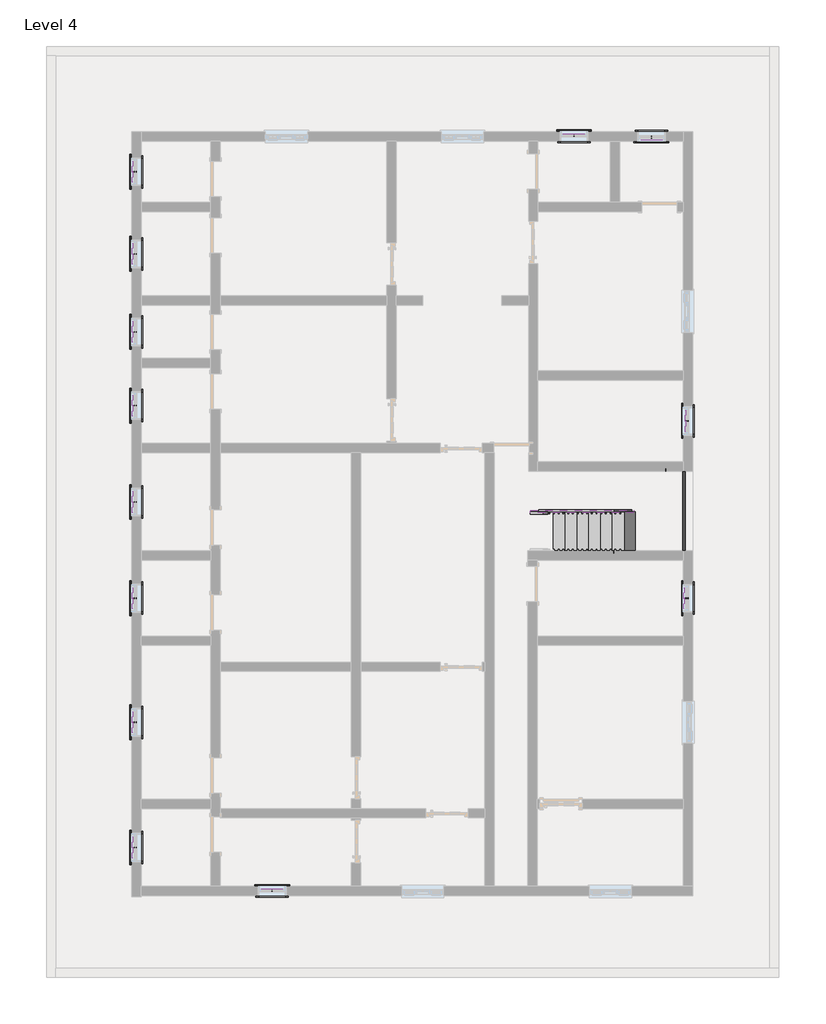
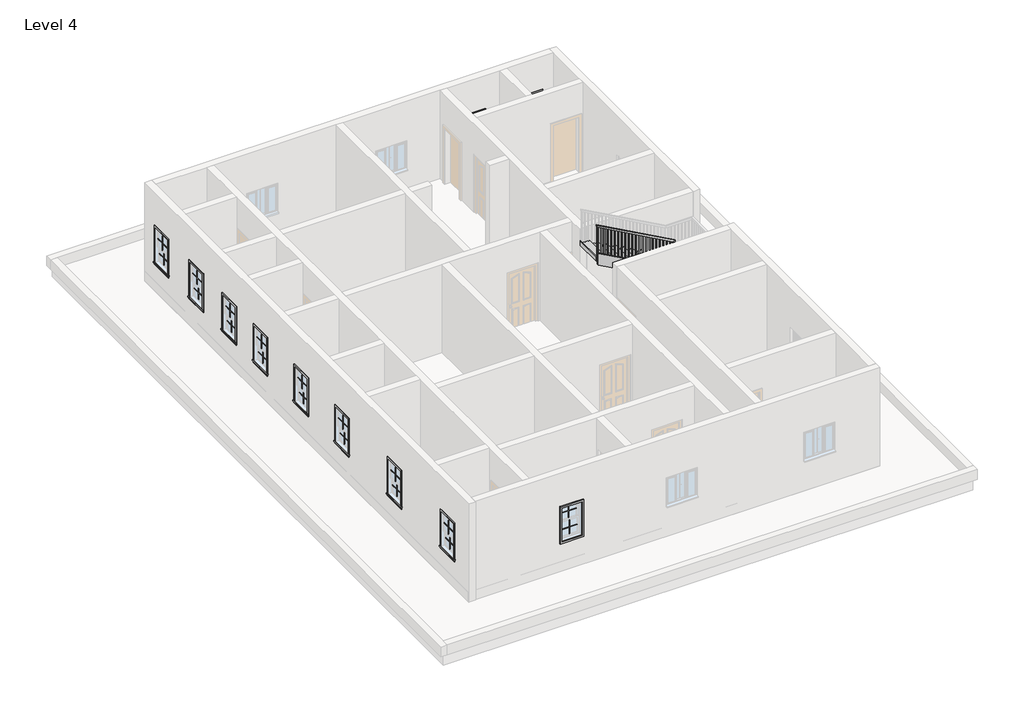
# One storey, part 3 of 3: 52 proxies, 5 members, 1 railing, 1 stair flight.
"""IFC4 building model written with IfcOpenShell, lengths in millimetres."""

from ifc_helpers import new_model, si_unit, frame, origin, place, context, project, spatial, polyline, outline, extrude, faceted_brep, transform, mapped, element, save
from components import muntin_pattern_2x2_muntin_pattern_2x2_eba6c5fb, trim_window_exterior_flat_with_sill_278e6a94, trim_window_interior_flat_picture_frame_e9fd5f45, stair_flight_f099b86a

model = new_model("IFC4")

# Units and contexts
model_context = context("Model", 3, world=origin())
ifc_project = project(units=[si_unit("LENGTHUNIT", "METRE", prefix="MILLI")], contexts=[model_context])

# Site, building, storey
site = spatial("IfcSite", under=ifc_project)
building = spatial("IfcBuilding", under=site)
storey = spatial("IfcBuildingStorey", under=building, Name="Level 4", Elevation=9144.0)

# Proxies
placement = place(None, origin())
muntin_pattern_2x2_muntin_pattern_2x2_shape = muntin_pattern_2x2_muntin_pattern_2x2_eba6c5fb(model_context)
element("IfcBuildingElementProxy", 1, Name="Muntin Pattern_2x2 : Muntin Pattern_2x2", ObjectType="Muntin Pattern_2x2 : Muntin Pattern_2x2", at=placement, inside=storey, context=model_context, shape_type="MappedRepresentation", body=[
    mapped(muntin_pattern_2x2_muntin_pattern_2x2_shape, transform((-10440.7626145, 6547.3404944, 10614.025), x_axis=(0.0, 1.0, 0.0), y_axis=(-1.0, 0.0, 0.0), z_axis=(0.0, 0.0, 1.0))),
])
element("IfcBuildingElementProxy", 2, Name="Muntin Pattern_2x2 : Muntin Pattern_2x2", ObjectType="Muntin Pattern_2x2 : Muntin Pattern_2x2", at=placement, inside=storey, context=model_context, shape_type="MappedRepresentation", body=[
    mapped(muntin_pattern_2x2_muntin_pattern_2x2_shape, transform((-10396.3126145, 6547.3404944, 10134.6), x_axis=(0.0, 1.0, 0.0), y_axis=(-1.0, 0.0, 0.0), z_axis=(0.0, 0.0, 1.0))),
])
element("IfcBuildingElementProxy", 3, Name="Muntin Pattern_2x2 : Muntin Pattern_2x2", ObjectType="Muntin Pattern_2x2 : Muntin Pattern_2x2", at=placement, inside=storey, context=model_context, shape_type="MappedRepresentation", body=[
    mapped(muntin_pattern_2x2_muntin_pattern_2x2_shape, transform((-10440.7626145, 4782.0404944, 10614.025), x_axis=(0.0, 1.0, 0.0), y_axis=(-1.0, 0.0, 0.0), z_axis=(0.0, 0.0, 1.0))),
])
element("IfcBuildingElementProxy", 4, Name="Muntin Pattern_2x2 : Muntin Pattern_2x2", ObjectType="Muntin Pattern_2x2 : Muntin Pattern_2x2", at=placement, inside=storey, context=model_context, shape_type="MappedRepresentation", body=[
    mapped(muntin_pattern_2x2_muntin_pattern_2x2_shape, transform((-10396.3126145, 4782.0404944, 10134.6), x_axis=(0.0, 1.0, 0.0), y_axis=(-1.0, 0.0, 0.0), z_axis=(0.0, 0.0, 1.0))),
])
element("IfcBuildingElementProxy", 5, Name="Muntin Pattern_2x2 : Muntin Pattern_2x2", ObjectType="Muntin Pattern_2x2 : Muntin Pattern_2x2", at=placement, inside=storey, context=model_context, shape_type="MappedRepresentation", body=[
    mapped(muntin_pattern_2x2_muntin_pattern_2x2_shape, transform((-10440.7626145, 3105.6404944, 10614.025), x_axis=(0.0, 1.0, 0.0), y_axis=(-1.0, 0.0, 0.0), z_axis=(0.0, 0.0, 1.0))),
])
element("IfcBuildingElementProxy", 6, Name="Muntin Pattern_2x2 : Muntin Pattern_2x2", ObjectType="Muntin Pattern_2x2 : Muntin Pattern_2x2", at=placement, inside=storey, context=model_context, shape_type="MappedRepresentation", body=[
    mapped(muntin_pattern_2x2_muntin_pattern_2x2_shape, transform((-10396.3126145, 3105.6404944, 10134.6), x_axis=(0.0, 1.0, 0.0), y_axis=(-1.0, 0.0, 0.0), z_axis=(0.0, 0.0, 1.0))),
])
element("IfcBuildingElementProxy", 7, Name="Muntin Pattern_2x2 : Muntin Pattern_2x2", ObjectType="Muntin Pattern_2x2 : Muntin Pattern_2x2", at=placement, inside=storey, context=model_context, shape_type="MappedRepresentation", body=[
    mapped(muntin_pattern_2x2_muntin_pattern_2x2_shape, transform((-10440.7626145, 1518.1404944, 10614.025), x_axis=(0.0, 1.0, 0.0), y_axis=(-1.0, 0.0, 0.0), z_axis=(0.0, 0.0, 1.0))),
])
element("IfcBuildingElementProxy", 8, Name="Muntin Pattern_2x2 : Muntin Pattern_2x2", ObjectType="Muntin Pattern_2x2 : Muntin Pattern_2x2", at=placement, inside=storey, context=model_context, shape_type="MappedRepresentation", body=[
    mapped(muntin_pattern_2x2_muntin_pattern_2x2_shape, transform((-10396.3126145, 1518.1404944, 10134.6), x_axis=(0.0, 1.0, 0.0), y_axis=(-1.0, 0.0, 0.0), z_axis=(0.0, 0.0, 1.0))),
])
element("IfcBuildingElementProxy", 9, Name="Muntin Pattern_2x2 : Muntin Pattern_2x2", ObjectType="Muntin Pattern_2x2 : Muntin Pattern_2x2", at=placement, inside=storey, context=model_context, shape_type="MappedRepresentation", body=[
    mapped(muntin_pattern_2x2_muntin_pattern_2x2_shape, transform((-10440.7626145, -551.9595056, 10614.025), x_axis=(0.0, 1.0, 0.0), y_axis=(-1.0, 0.0, 0.0), z_axis=(0.0, 0.0, 1.0))),
])
element("IfcBuildingElementProxy", 10, Name="Muntin Pattern_2x2 : Muntin Pattern_2x2", ObjectType="Muntin Pattern_2x2 : Muntin Pattern_2x2", at=placement, inside=storey, context=model_context, shape_type="MappedRepresentation", body=[
    mapped(muntin_pattern_2x2_muntin_pattern_2x2_shape, transform((-10396.3126145, -551.9595056, 10134.6), x_axis=(0.0, 1.0, 0.0), y_axis=(-1.0, 0.0, 0.0), z_axis=(0.0, 0.0, 1.0))),
])
element("IfcBuildingElementProxy", 11, Name="Muntin Pattern_2x2 : Muntin Pattern_2x2", ObjectType="Muntin Pattern_2x2 : Muntin Pattern_2x2", at=placement, inside=storey, context=model_context, shape_type="MappedRepresentation", body=[
    mapped(muntin_pattern_2x2_muntin_pattern_2x2_shape, transform((-10440.7626145, -2622.0595056, 10614.025), x_axis=(0.0, 1.0, 0.0), y_axis=(-1.0, 0.0, 0.0), z_axis=(0.0, 0.0, 1.0))),
])
element("IfcBuildingElementProxy", 12, Name="Muntin Pattern_2x2 : Muntin Pattern_2x2", ObjectType="Muntin Pattern_2x2 : Muntin Pattern_2x2", at=placement, inside=storey, context=model_context, shape_type="MappedRepresentation", body=[
    mapped(muntin_pattern_2x2_muntin_pattern_2x2_shape, transform((-10396.3126145, -2622.0595056, 10134.6), x_axis=(0.0, 1.0, 0.0), y_axis=(-1.0, 0.0, 0.0), z_axis=(0.0, 0.0, 1.0))),
])
element("IfcBuildingElementProxy", 13, Name="Muntin Pattern_2x2 : Muntin Pattern_2x2", ObjectType="Muntin Pattern_2x2 : Muntin Pattern_2x2", at=placement, inside=storey, context=model_context, shape_type="MappedRepresentation", body=[
    mapped(muntin_pattern_2x2_muntin_pattern_2x2_shape, transform((-10440.7626145, -5289.0595056, 10614.025), x_axis=(0.0, 1.0, 0.0), y_axis=(-1.0, 0.0, 0.0), z_axis=(0.0, 0.0, 1.0))),
])
element("IfcBuildingElementProxy", 14, Name="Muntin Pattern_2x2 : Muntin Pattern_2x2", ObjectType="Muntin Pattern_2x2 : Muntin Pattern_2x2", at=placement, inside=storey, context=model_context, shape_type="MappedRepresentation", body=[
    mapped(muntin_pattern_2x2_muntin_pattern_2x2_shape, transform((-10396.3126145, -5289.0595056, 10134.6), x_axis=(0.0, 1.0, 0.0), y_axis=(-1.0, 0.0, 0.0), z_axis=(0.0, 0.0, 1.0))),
])
element("IfcBuildingElementProxy", 15, Name="Muntin Pattern_2x2 : Muntin Pattern_2x2", ObjectType="Muntin Pattern_2x2 : Muntin Pattern_2x2", at=placement, inside=storey, context=model_context, shape_type="MappedRepresentation", body=[
    mapped(muntin_pattern_2x2_muntin_pattern_2x2_shape, transform((-10440.7626145, -7981.4595056, 10614.025), x_axis=(0.0, 1.0, 0.0), y_axis=(-1.0, 0.0, 0.0), z_axis=(0.0, 0.0, 1.0))),
])
element("IfcBuildingElementProxy", 16, Name="Muntin Pattern_2x2 : Muntin Pattern_2x2", ObjectType="Muntin Pattern_2x2 : Muntin Pattern_2x2", at=placement, inside=storey, context=model_context, shape_type="MappedRepresentation", body=[
    mapped(muntin_pattern_2x2_muntin_pattern_2x2_shape, transform((-10396.3126145, -7981.4595056, 10134.6), x_axis=(0.0, 1.0, 0.0), y_axis=(-1.0, 0.0, 0.0), z_axis=(0.0, 0.0, 1.0))),
])
element("IfcBuildingElementProxy", 17, Name="Muntin Pattern_2x2 : Muntin Pattern_2x2", ObjectType="Muntin Pattern_2x2 : Muntin Pattern_2x2", at=placement, inside=storey, context=model_context, shape_type="MappedRepresentation", body=[
    mapped(muntin_pattern_2x2_muntin_pattern_2x2_shape, transform((-7453.0876145, -8854.5845056, 10614.025), x_axis=(1.0, 0.0, 0.0), y_axis=(0.0, 1.0, 0.0), z_axis=(0.0, 0.0, 1.0))),
])
element("IfcBuildingElementProxy", 18, Name="Muntin Pattern_2x2 : Muntin Pattern_2x2", ObjectType="Muntin Pattern_2x2 : Muntin Pattern_2x2", at=placement, inside=storey, context=model_context, shape_type="MappedRepresentation", body=[
    mapped(muntin_pattern_2x2_muntin_pattern_2x2_shape, transform((-7453.0876145, -8899.0345056, 10134.6), x_axis=(1.0, 0.0, 0.0), y_axis=(0.0, 1.0, 0.0), z_axis=(0.0, 0.0, 1.0))),
])
element("IfcBuildingElementProxy", 19, Name="Muntin Pattern_2x2 : Muntin Pattern_2x2", ObjectType="Muntin Pattern_2x2 : Muntin Pattern_2x2", at=placement, inside=storey, context=model_context, shape_type="MappedRepresentation", body=[
    mapped(muntin_pattern_2x2_muntin_pattern_2x2_shape, transform((1421.0373855, -2622.0595056, 10614.025), x_axis=(0.0, 1.0, 0.0), y_axis=(-1.0, 0.0, 0.0), z_axis=(0.0, 0.0, 1.0))),
])
element("IfcBuildingElementProxy", 20, Name="Muntin Pattern_2x2 : Muntin Pattern_2x2", ObjectType="Muntin Pattern_2x2 : Muntin Pattern_2x2", at=placement, inside=storey, context=model_context, shape_type="MappedRepresentation", body=[
    mapped(muntin_pattern_2x2_muntin_pattern_2x2_shape, transform((1465.4873855, -2622.0595056, 10134.6), x_axis=(0.0, 1.0, 0.0), y_axis=(-1.0, 0.0, 0.0), z_axis=(0.0, 0.0, 1.0))),
])
element("IfcBuildingElementProxy", 21, Name="Muntin Pattern_2x2 : Muntin Pattern_2x2", ObjectType="Muntin Pattern_2x2 : Muntin Pattern_2x2", at=placement, inside=storey, context=model_context, shape_type="MappedRepresentation", body=[
    mapped(muntin_pattern_2x2_muntin_pattern_2x2_shape, transform((1421.0373855, 1190.4645364, 10614.025), x_axis=(0.0, 1.0, 0.0), y_axis=(-1.0, 0.0, 0.0), z_axis=(0.0, 0.0, 1.0))),
])
element("IfcBuildingElementProxy", 22, Name="Muntin Pattern_2x2 : Muntin Pattern_2x2", ObjectType="Muntin Pattern_2x2 : Muntin Pattern_2x2", at=placement, inside=storey, context=model_context, shape_type="MappedRepresentation", body=[
    mapped(muntin_pattern_2x2_muntin_pattern_2x2_shape, transform((1465.4873855, 1190.4645364, 10134.6), x_axis=(0.0, 1.0, 0.0), y_axis=(-1.0, 0.0, 0.0), z_axis=(0.0, 0.0, 1.0))),
])
element("IfcBuildingElementProxy", 23, Name="Muntin Pattern_2x2 : Muntin Pattern_2x2", ObjectType="Muntin Pattern_2x2 : Muntin Pattern_2x2", at=placement, inside=storey, context=model_context, shape_type="MappedRepresentation", body=[
    mapped(muntin_pattern_2x2_muntin_pattern_2x2_shape, transform((700.3123855, 7242.6654944, 10614.025), x_axis=(-1.0, 0.0, 0.0), y_axis=(0.0, -1.0, 0.0), z_axis=(0.0, 0.0, 1.0))),
])
element("IfcBuildingElementProxy", 24, Name="Muntin Pattern_2x2 : Muntin Pattern_2x2", ObjectType="Muntin Pattern_2x2 : Muntin Pattern_2x2", at=placement, inside=storey, context=model_context, shape_type="MappedRepresentation", body=[
    mapped(muntin_pattern_2x2_muntin_pattern_2x2_shape, transform((700.3123855, 7287.1154944, 10134.6), x_axis=(-1.0, 0.0, 0.0), y_axis=(0.0, -1.0, 0.0), z_axis=(0.0, 0.0, 1.0))),
])
element("IfcBuildingElementProxy", 25, Name="Muntin Pattern_2x2 : Muntin Pattern_2x2", ObjectType="Muntin Pattern_2x2 : Muntin Pattern_2x2", at=placement, inside=storey, context=model_context, shape_type="MappedRepresentation", body=[
    mapped(muntin_pattern_2x2_muntin_pattern_2x2_shape, transform((-963.3876145, 7376.0154944, 10614.025), x_axis=(1.0, 0.0, 0.0), y_axis=(0.0, 1.0, 0.0), z_axis=(0.0, 0.0, 1.0))),
])
element("IfcBuildingElementProxy", 26, Name="Muntin Pattern_2x2 : Muntin Pattern_2x2", ObjectType="Muntin Pattern_2x2 : Muntin Pattern_2x2", at=placement, inside=storey, context=model_context, shape_type="MappedRepresentation", body=[
    mapped(muntin_pattern_2x2_muntin_pattern_2x2_shape, transform((-963.3876145, 7331.5654944, 10134.6), x_axis=(1.0, 0.0, 0.0), y_axis=(0.0, 1.0, 0.0), z_axis=(0.0, 0.0, 1.0))),
])
trim_window_exterior_flat_with_sill_shape = trim_window_exterior_flat_with_sill_278e6a94(model_context)
element("IfcBuildingElementProxy", 27, Name="Trim-Window-Exterior-Flat : with Sill", ObjectType="Trim-Window-Exterior-Flat : with Sill", at=placement, inside=storey, context=model_context, shape_type="MappedRepresentation", body=[
    mapped(trim_window_exterior_flat_with_sill_shape, transform((-10475.6876145, 6547.3404944, 11125.2), x_axis=(0.0, -1.0, 0.0), y_axis=(0.0, 0.0, 1.0), z_axis=(-1.0, 0.0, 0.0))),
])
element("IfcBuildingElementProxy", 28, Name="Trim-Window-Exterior-Flat : with Sill", ObjectType="Trim-Window-Exterior-Flat : with Sill", at=placement, inside=storey, context=model_context, shape_type="MappedRepresentation", body=[
    mapped(trim_window_exterior_flat_with_sill_shape, transform((-10475.6876145, 4782.0404944, 11125.2), x_axis=(0.0, -1.0, 0.0), y_axis=(0.0, 0.0, 1.0), z_axis=(-1.0, 0.0, 0.0))),
])
element("IfcBuildingElementProxy", 29, Name="Trim-Window-Exterior-Flat : with Sill", ObjectType="Trim-Window-Exterior-Flat : with Sill", at=placement, inside=storey, context=model_context, shape_type="MappedRepresentation", body=[
    mapped(trim_window_exterior_flat_with_sill_shape, transform((-10475.6876145, 3105.6404944, 11125.2), x_axis=(0.0, -1.0, 0.0), y_axis=(0.0, 0.0, 1.0), z_axis=(-1.0, 0.0, 0.0))),
])
element("IfcBuildingElementProxy", 30, Name="Trim-Window-Exterior-Flat : with Sill", ObjectType="Trim-Window-Exterior-Flat : with Sill", at=placement, inside=storey, context=model_context, shape_type="MappedRepresentation", body=[
    mapped(trim_window_exterior_flat_with_sill_shape, transform((-10475.6876145, 1518.1404944, 11125.2), x_axis=(0.0, -1.0, 0.0), y_axis=(0.0, 0.0, 1.0), z_axis=(-1.0, 0.0, 0.0))),
])
element("IfcBuildingElementProxy", 31, Name="Trim-Window-Exterior-Flat : with Sill", ObjectType="Trim-Window-Exterior-Flat : with Sill", at=placement, inside=storey, context=model_context, shape_type="MappedRepresentation", body=[
    mapped(trim_window_exterior_flat_with_sill_shape, transform((-10475.6876145, -551.9595056, 11125.2), x_axis=(0.0, -1.0, 0.0), y_axis=(0.0, 0.0, 1.0), z_axis=(-1.0, 0.0, 0.0))),
])
element("IfcBuildingElementProxy", 32, Name="Trim-Window-Exterior-Flat : with Sill", ObjectType="Trim-Window-Exterior-Flat : with Sill", at=placement, inside=storey, context=model_context, shape_type="MappedRepresentation", body=[
    mapped(trim_window_exterior_flat_with_sill_shape, transform((-10475.6876145, -2622.0595056, 11125.2), x_axis=(0.0, -1.0, 0.0), y_axis=(0.0, 0.0, 1.0), z_axis=(-1.0, 0.0, 0.0))),
])
element("IfcBuildingElementProxy", 33, Name="Trim-Window-Exterior-Flat : with Sill", ObjectType="Trim-Window-Exterior-Flat : with Sill", at=placement, inside=storey, context=model_context, shape_type="MappedRepresentation", body=[
    mapped(trim_window_exterior_flat_with_sill_shape, transform((-10475.6876145, -5289.0595056, 11125.2), x_axis=(0.0, -1.0, 0.0), y_axis=(0.0, 0.0, 1.0), z_axis=(-1.0, 0.0, 0.0))),
])
element("IfcBuildingElementProxy", 34, Name="Trim-Window-Exterior-Flat : with Sill", ObjectType="Trim-Window-Exterior-Flat : with Sill", at=placement, inside=storey, context=model_context, shape_type="MappedRepresentation", body=[
    mapped(trim_window_exterior_flat_with_sill_shape, transform((-10475.6876145, -7981.4595056, 11125.2), x_axis=(0.0, -1.0, 0.0), y_axis=(0.0, 0.0, 1.0), z_axis=(-1.0, 0.0, 0.0))),
])
element("IfcBuildingElementProxy", 35, Name="Trim-Window-Exterior-Flat : with Sill", ObjectType="Trim-Window-Exterior-Flat : with Sill", at=placement, inside=storey, context=model_context, shape_type="MappedRepresentation", body=[
    mapped(trim_window_exterior_flat_with_sill_shape, transform((-7453.0876145, -8819.6595056, 11125.2), x_axis=(-1.0, 0.0, 0.0), y_axis=(0.0, 0.0, 1.0), z_axis=(0.0, 1.0, 0.0))),
])
element("IfcBuildingElementProxy", 36, Name="Trim-Window-Exterior-Flat : with Sill", ObjectType="Trim-Window-Exterior-Flat : with Sill", at=placement, inside=storey, context=model_context, shape_type="MappedRepresentation", body=[
    mapped(trim_window_exterior_flat_with_sill_shape, transform((1386.1123855, -2622.0595056, 11125.2), x_axis=(0.0, -1.0, 0.0), y_axis=(0.0, 0.0, 1.0), z_axis=(-1.0, 0.0, 0.0))),
])
element("IfcBuildingElementProxy", 37, Name="Trim-Window-Exterior-Flat : with Sill", ObjectType="Trim-Window-Exterior-Flat : with Sill", at=placement, inside=storey, context=model_context, shape_type="MappedRepresentation", body=[
    mapped(trim_window_exterior_flat_with_sill_shape, transform((1386.1123855, 1190.4645364, 11125.2), x_axis=(0.0, -1.0, 0.0), y_axis=(0.0, 0.0, 1.0), z_axis=(-1.0, 0.0, 0.0))),
])
element("IfcBuildingElementProxy", 38, Name="Trim-Window-Exterior-Flat : with Sill", ObjectType="Trim-Window-Exterior-Flat : with Sill", at=placement, inside=storey, context=model_context, shape_type="MappedRepresentation", body=[
    mapped(trim_window_exterior_flat_with_sill_shape, transform((700.3123855, 7207.7404944, 11125.2), x_axis=(1.0, 0.0, 0.0), y_axis=(0.0, 0.0, 1.0), z_axis=(0.0, -1.0, 0.0))),
])
element("IfcBuildingElementProxy", 39, Name="Trim-Window-Exterior-Flat : with Sill", ObjectType="Trim-Window-Exterior-Flat : with Sill", at=placement, inside=storey, context=model_context, shape_type="MappedRepresentation", body=[
    mapped(trim_window_exterior_flat_with_sill_shape, transform((-963.3876145, 7410.9404944, 11125.2), x_axis=(-1.0, 0.0, 0.0), y_axis=(0.0, 0.0, 1.0), z_axis=(0.0, 1.0, 0.0))),
])
trim_window_interior_flat_picture_frame_shape = trim_window_interior_flat_picture_frame_e9fd5f45(model_context)
element("IfcBuildingElementProxy", 40, Name="Trim-Window-Interior-Flat : Picture Frame", ObjectType="Trim-Window-Interior-Flat : Picture Frame", at=placement, inside=storey, context=model_context, shape_type="MappedRepresentation", body=[
    mapped(trim_window_interior_flat_picture_frame_shape, transform((-10272.4876145, 6547.3404944, 11125.2), x_axis=(0.0, 1.0, 0.0), y_axis=(0.0, 0.0, 1.0), z_axis=(1.0, 0.0, 0.0))),
])
element("IfcBuildingElementProxy", 41, Name="Trim-Window-Interior-Flat : Picture Frame", ObjectType="Trim-Window-Interior-Flat : Picture Frame", at=placement, inside=storey, context=model_context, shape_type="MappedRepresentation", body=[
    mapped(trim_window_interior_flat_picture_frame_shape, transform((-10272.4876145, 4782.0404944, 11125.2), x_axis=(0.0, 1.0, 0.0), y_axis=(0.0, 0.0, 1.0), z_axis=(1.0, 0.0, 0.0))),
])
element("IfcBuildingElementProxy", 42, Name="Trim-Window-Interior-Flat : Picture Frame", ObjectType="Trim-Window-Interior-Flat : Picture Frame", at=placement, inside=storey, context=model_context, shape_type="MappedRepresentation", body=[
    mapped(trim_window_interior_flat_picture_frame_shape, transform((-10272.4876145, 3105.6404944, 11125.2), x_axis=(0.0, 1.0, 0.0), y_axis=(0.0, 0.0, 1.0), z_axis=(1.0, 0.0, 0.0))),
])
element("IfcBuildingElementProxy", 43, Name="Trim-Window-Interior-Flat : Picture Frame", ObjectType="Trim-Window-Interior-Flat : Picture Frame", at=placement, inside=storey, context=model_context, shape_type="MappedRepresentation", body=[
    mapped(trim_window_interior_flat_picture_frame_shape, transform((-10272.4876145, 1518.1404944, 11125.2), x_axis=(0.0, 1.0, 0.0), y_axis=(0.0, 0.0, 1.0), z_axis=(1.0, 0.0, 0.0))),
])
element("IfcBuildingElementProxy", 44, Name="Trim-Window-Interior-Flat : Picture Frame", ObjectType="Trim-Window-Interior-Flat : Picture Frame", at=placement, inside=storey, context=model_context, shape_type="MappedRepresentation", body=[
    mapped(trim_window_interior_flat_picture_frame_shape, transform((-10272.4876145, -551.9595056, 11125.2), x_axis=(0.0, 1.0, 0.0), y_axis=(0.0, 0.0, 1.0), z_axis=(1.0, 0.0, 0.0))),
])
element("IfcBuildingElementProxy", 45, Name="Trim-Window-Interior-Flat : Picture Frame", ObjectType="Trim-Window-Interior-Flat : Picture Frame", at=placement, inside=storey, context=model_context, shape_type="MappedRepresentation", body=[
    mapped(trim_window_interior_flat_picture_frame_shape, transform((-10272.4876145, -2622.0595056, 11125.2), x_axis=(0.0, 1.0, 0.0), y_axis=(0.0, 0.0, 1.0), z_axis=(1.0, 0.0, 0.0))),
])
element("IfcBuildingElementProxy", 46, Name="Trim-Window-Interior-Flat : Picture Frame", ObjectType="Trim-Window-Interior-Flat : Picture Frame", at=placement, inside=storey, context=model_context, shape_type="MappedRepresentation", body=[
    mapped(trim_window_interior_flat_picture_frame_shape, transform((-10272.4876145, -5289.0595056, 11125.2), x_axis=(0.0, 1.0, 0.0), y_axis=(0.0, 0.0, 1.0), z_axis=(1.0, 0.0, 0.0))),
])
element("IfcBuildingElementProxy", 47, Name="Trim-Window-Interior-Flat : Picture Frame", ObjectType="Trim-Window-Interior-Flat : Picture Frame", at=placement, inside=storey, context=model_context, shape_type="MappedRepresentation", body=[
    mapped(trim_window_interior_flat_picture_frame_shape, transform((-10272.4876145, -7981.4595056, 11125.2), x_axis=(0.0, 1.0, 0.0), y_axis=(0.0, 0.0, 1.0), z_axis=(1.0, 0.0, 0.0))),
])
element("IfcBuildingElementProxy", 48, Name="Trim-Window-Interior-Flat : Picture Frame", ObjectType="Trim-Window-Interior-Flat : Picture Frame", at=placement, inside=storey, context=model_context, shape_type="MappedRepresentation", body=[
    mapped(trim_window_interior_flat_picture_frame_shape, transform((-7453.0876145, -9022.8595056, 11125.2), x_axis=(1.0, 0.0, 0.0), y_axis=(0.0, 0.0, 1.0), z_axis=(0.0, -1.0, 0.0))),
])
element("IfcBuildingElementProxy", 49, Name="Trim-Window-Interior-Flat : Picture Frame", ObjectType="Trim-Window-Interior-Flat : Picture Frame", at=placement, inside=storey, context=model_context, shape_type="MappedRepresentation", body=[
    mapped(trim_window_interior_flat_picture_frame_shape, transform((1589.3123855, -2622.0595056, 11125.2), x_axis=(0.0, 1.0, 0.0), y_axis=(0.0, 0.0, 1.0), z_axis=(1.0, 0.0, 0.0))),
])
element("IfcBuildingElementProxy", 50, Name="Trim-Window-Interior-Flat : Picture Frame", ObjectType="Trim-Window-Interior-Flat : Picture Frame", at=placement, inside=storey, context=model_context, shape_type="MappedRepresentation", body=[
    mapped(trim_window_interior_flat_picture_frame_shape, transform((1589.3123855, 1190.4645364, 11125.2), x_axis=(0.0, 1.0, 0.0), y_axis=(0.0, 0.0, 1.0), z_axis=(1.0, 0.0, 0.0))),
])
element("IfcBuildingElementProxy", 51, Name="Trim-Window-Interior-Flat : Picture Frame", ObjectType="Trim-Window-Interior-Flat : Picture Frame", at=placement, inside=storey, context=model_context, shape_type="MappedRepresentation", body=[
    mapped(trim_window_interior_flat_picture_frame_shape, transform((700.3123855, 7410.9404944, 11125.2), x_axis=(-1.0, 0.0, 0.0), y_axis=(0.0, 0.0, 1.0), z_axis=(0.0, 1.0, 0.0))),
])
element("IfcBuildingElementProxy", 52, Name="Trim-Window-Interior-Flat : Picture Frame", ObjectType="Trim-Window-Interior-Flat : Picture Frame", at=placement, inside=storey, context=model_context, shape_type="MappedRepresentation", body=[
    mapped(trim_window_interior_flat_picture_frame_shape, transform((-963.3876145, 7207.7404944, 11125.2), x_axis=(1.0, 0.0, 0.0), y_axis=(0.0, 0.0, 1.0), z_axis=(0.0, -1.0, 0.0))),
])

# Members
element("IfcMember", 53, ObjectType="Stringer - 2\" Width", at=placement, inside=storey, context=model_context, shape_type="SweptSolid", body=[
    extrude(outline(polyline([(9354.6757607, -1903.1876145), (9144.0, -1903.1876145), (9144.0, -1654.2050647), (10209.4963497, 274.6830625), (10557.7073019, 274.6830625), (9354.6757607, -1903.1876145)])), frame((0.0, -767.8595056, 0.0), z_axis=(0.0, 1.0, 0.0), x_axis=(0.0, 0.0, 1.0)), (0.0, 0.0, 1.0), 50.8),
])
element("IfcMember", 54, ObjectType="Stringer - 2\" Width", at=placement, inside=storey, context=model_context, shape_type="SweptSolid", body=[
    extrude(outline(polyline([(10374.7177047, 325.4830625), (10722.928657, 325.4830625), (11954.0215532, -1903.1876145), (11605.8106009, -1903.1876145), (10374.7177047, 325.4830625)])), frame((0.0, -780.5595056, 0.0), z_axis=(0.0, 1.0, 0.0), x_axis=(0.0, 0.0, 1.0)), (0.0, 0.0, 1.0), 50.8),
])
element("IfcMember", 55, ObjectType="Stringer - 2\" Width", at=placement, inside=storey, context=model_context, shape_type="SweptSolid", body=[
    extrude(outline(polyline([(9354.6757607, -1903.1876145), (9144.0, -1903.1876145), (9144.0, -1654.2050647), (10591.8, 966.7745674), (10591.8, 336.4017165), (9354.6757607, -1903.1876145)])), frame((0.0, -1656.8595056, 0.0), z_axis=(0.0, 1.0, 0.0), x_axis=(0.0, 0.0, 1.0)), (0.0, 0.0, 1.0), 50.8),
])
element("IfcMember", 56, ObjectType="Stringer - 2\" Width", at=placement, inside=storey, context=model_context, shape_type="SweptSolid", body=[
    extrude(outline(polyline([(1424.2123855, -1656.8595056), (1373.4123855, -1656.8595056), (1373.4123855, 108.4404944), (1424.2123855, 108.4404944), (1424.2123855, -1656.8595056)])), frame((0.0, 0.0, 10287.0), z_axis=(0.0, 0.0, 1.0), x_axis=(1.0, 0.0, 0.0)), (0.0, 0.0, 1.0), 304.8),
])
element("IfcMember", 57, ObjectType="Stringer - 2\" Width", at=placement, inside=storey, context=model_context, shape_type="SweptSolid", body=[
    extrude(outline(polyline([(10287.0, 1114.6529278), (11954.0215532, -1903.1876145), (11605.8106009, -1903.1876145), (10287.0, 484.2800769), (10287.0, 1114.6529278)])), frame((0.0, 108.4404944, 0.0), z_axis=(0.0, 1.0, 0.0), x_axis=(0.0, 0.0, 1.0)), (0.0, 0.0, 1.0), 50.8),
])

# Railing
element("IfcRailing", 58, ObjectType="Handrail - Rectangular", at=placement, inside=storey, context=model_context, shape_type="SolidModel", body=[
    faceted_brep([(-1903.1876145, -767.8595056, 10195.56), (-1903.1876145, -767.8595056, 10137.4879132), (-1903.1876145, -818.6595056, 10137.4879132), (-1903.1876145, -818.6595056, 10195.56), (325.4830625, -767.8595056, 11430.0), (325.4830625, -818.6595056, 11430.0), (325.4830625, -818.6595056, 11371.9279132), (325.4830625, -767.8595056, 11371.9279132)], [[[0, 1, 2, 3]], [[4, 5, 6, 7]], [[1, 0, 4, 7]], [[2, 1, 7, 6]], [[3, 2, 6, 5]], [[0, 3, 5, 4]]]),
    faceted_brep([(325.4830625, -818.6595056, 11430.0), (325.4830625, -818.6595056, 11379.2), (376.2830625, -818.6595056, 11379.2), (376.2830625, -818.6595056, 11430.0), (325.4830625, -729.7595056, 11430.0), (376.2830625, -729.7595056, 11430.0), (376.2830625, -678.9595056, 11379.2), (325.4830625, -678.9595056, 11379.2)], [[[0, 1, 2, 3]], [[4, 5, 6, 7]], [[1, 0, 4, 7]], [[2, 1, 7, 6]], [[3, 2, 6, 5]], [[0, 3, 5, 4]]]),
    faceted_brep([(325.4830625, -729.7595056, 11430.0), (325.4830625, -678.9595056, 11379.2), (376.2830625, -678.9595056, 11379.2), (376.2830625, -729.7595056, 11430.0), (325.4830625, -729.7595056, 11509.0879132), (376.2830625, -729.7595056, 11539.0223516), (376.2830625, -678.9595056, 11539.0223516), (325.4830625, -678.9595056, 11509.0879132)], [[[0, 1, 2, 3]], [[4, 5, 6, 7]], [[1, 0, 4, 7]], [[2, 1, 7, 6]], [[3, 2, 6, 5]], [[0, 3, 5, 4]]]),
    faceted_brep([(376.2830625, -729.7595056, 11539.0223516), (325.4830625, -729.7595056, 11509.0879132), (325.4830625, -678.9595056, 11509.0879132), (376.2830625, -678.9595056, 11539.0223516), (-1903.1876145, -729.7595056, 12801.6), (-1903.1876145, -678.9595056, 12801.6), (-1903.1876145, -678.9595056, 12743.5279132), (-1903.1876145, -729.7595056, 12743.5279132)], [[[0, 1, 2, 3]], [[4, 5, 6, 7]], [[1, 0, 4, 7]], [[2, 1, 7, 6]], [[3, 2, 6, 5]], [[0, 3, 5, 4]]]),
    extrude(outline(polyline([(12738.3072849, -1893.8419375), (11750.04, -1893.8419375), (11750.04, -1874.7919375), (12727.7556667, -1874.7919375), (12738.3072849, -1893.8419375)])), frame((0.0, -713.8845056, 0.0), z_axis=(0.0, 1.0, 0.0), x_axis=(0.0, 0.0, 1.0)), (0.0, 0.0, 1.0), 19.05),
    extrude(outline(polyline([(12682.031988, -1792.2419375), (11750.04, -1792.2419375), (11750.04, -1773.1919375), (12671.4803699, -1773.1919375), (12682.031988, -1792.2419375)])), frame((0.0, -713.8845056, 0.0), z_axis=(0.0, 1.0, 0.0), x_axis=(0.0, 0.0, 1.0)), (0.0, 0.0, 1.0), 19.05),
    extrude(outline(polyline([(12625.7125465, -1690.6419375), (11750.04, -1690.6419375), (11750.04, -1671.5919375), (12615.1609284, -1671.5919375), (12625.7125465, -1690.6419375)])), frame((0.0, -713.8845056, 0.0), z_axis=(0.0, 1.0, 0.0), x_axis=(0.0, 0.0, 1.0)), (0.0, 0.0, 1.0), 19.05),
    extrude(outline(polyline([(12569.4813943, -1589.0419375), (11612.88, -1589.0419375), (11612.88, -1569.9919375), (12558.9297761, -1569.9919375), (12569.4813943, -1589.0419375)])), frame((0.0, -713.8845056, 0.0), z_axis=(0.0, 1.0, 0.0), x_axis=(0.0, 0.0, 1.0)), (0.0, 0.0, 1.0), 19.05),
    extrude(outline(polyline([(12513.2060974, -1487.4419375), (11612.88, -1487.4419375), (11612.88, -1468.3919375), (12502.6544792, -1468.3919375), (12513.2060974, -1487.4419375)])), frame((0.0, -713.8845056, 0.0), z_axis=(0.0, 1.0, 0.0), x_axis=(0.0, 0.0, 1.0)), (0.0, 0.0, 1.0), 19.05),
    extrude(outline(polyline([(12456.9308005, -1385.8419375), (11475.72, -1385.8419375), (11475.72, -1366.7919375), (12446.3791823, -1366.7919375), (12456.9308005, -1385.8419375)])), frame((0.0, -713.8845056, 0.0), z_axis=(0.0, 1.0, 0.0), x_axis=(0.0, 0.0, 1.0)), (0.0, 0.0, 1.0), 19.05),
    extrude(outline(polyline([(12400.6555036, -1284.2419375), (11475.72, -1284.2419375), (11475.72, -1265.1919375), (12390.1038855, -1265.1919375), (12400.6555036, -1284.2419375)])), frame((0.0, -713.8845056, 0.0), z_axis=(0.0, 1.0, 0.0), x_axis=(0.0, 0.0, 1.0)), (0.0, 0.0, 1.0), 19.05),
    extrude(outline(polyline([(12344.3802067, -1182.6419375), (11475.72, -1182.6419375), (11475.72, -1163.5919375), (12333.8285886, -1163.5919375), (12344.3802067, -1182.6419375)])), frame((0.0, -713.8845056, 0.0), z_axis=(0.0, 1.0, 0.0), x_axis=(0.0, 0.0, 1.0)), (0.0, 0.0, 1.0), 19.05),
    extrude(outline(polyline([(12288.1049099, -1081.0419375), (11338.56, -1081.0419375), (11338.56, -1061.9919375), (12277.5532917, -1061.9919375), (12288.1049099, -1081.0419375)])), frame((0.0, -713.8845056, 0.0), z_axis=(0.0, 1.0, 0.0), x_axis=(0.0, 0.0, 1.0)), (0.0, 0.0, 1.0), 19.05),
    extrude(outline(polyline([(12231.829613, -979.4419375), (11338.56, -979.4419375), (11338.56, -960.3919375), (12221.2779948, -960.3919375), (12231.829613, -979.4419375)])), frame((0.0, -713.8845056, 0.0), z_axis=(0.0, 1.0, 0.0), x_axis=(0.0, 0.0, 1.0)), (0.0, 0.0, 1.0), 19.05),
    extrude(outline(polyline([(12175.5543161, -877.8419375), (11201.4, -877.8419375), (11201.4, -858.7919375), (12165.0026979, -858.7919375), (12175.5543161, -877.8419375)])), frame((0.0, -713.8845056, 0.0), z_axis=(0.0, 1.0, 0.0), x_axis=(0.0, 0.0, 1.0)), (0.0, 0.0, 1.0), 19.05),
    extrude(outline(polyline([(12119.2790192, -776.2419375), (11201.4, -776.2419375), (11201.4, -757.1919375), (12108.727401, -757.1919375), (12119.2790192, -776.2419375)])), frame((0.0, -713.8845056, 0.0), z_axis=(0.0, 1.0, 0.0), x_axis=(0.0, 0.0, 1.0)), (0.0, 0.0, 1.0), 19.05),
    extrude(outline(polyline([(12063.0478669, -674.6419375), (11201.4, -674.6419375), (11201.4, -655.5919375), (12052.4962488, -655.5919375), (12063.0478669, -674.6419375)])), frame((0.0, -713.8845056, 0.0), z_axis=(0.0, 1.0, 0.0), x_axis=(0.0, 0.0, 1.0)), (0.0, 0.0, 1.0), 19.05),
    extrude(outline(polyline([(12006.77257, -573.0419375), (11064.24, -573.0419375), (11064.24, -553.9919375), (11996.2209519, -553.9919375), (12006.77257, -573.0419375)])), frame((0.0, -713.8845056, 0.0), z_axis=(0.0, 1.0, 0.0), x_axis=(0.0, 0.0, 1.0)), (0.0, 0.0, 1.0), 19.05),
    extrude(outline(polyline([(11950.4972732, -471.4419375), (11064.24, -471.4419375), (11064.24, -452.3919375), (11939.945655, -452.3919375), (11950.4972732, -471.4419375)])), frame((0.0, -713.8845056, 0.0), z_axis=(0.0, 1.0, 0.0), x_axis=(0.0, 0.0, 1.0)), (0.0, 0.0, 1.0), 19.05),
    extrude(outline(polyline([(11894.2219763, -369.8419375), (10927.08, -369.8419375), (10927.08, -350.7919375), (11883.6703581, -350.7919375), (11894.2219763, -369.8419375)])), frame((0.0, -713.8845056, 0.0), z_axis=(0.0, 1.0, 0.0), x_axis=(0.0, 0.0, 1.0)), (0.0, 0.0, 1.0), 19.05),
    extrude(outline(polyline([(11837.9466794, -268.2419375), (10927.08, -268.2419375), (10927.08, -249.1919375), (11827.3950612, -249.1919375), (11837.9466794, -268.2419375)])), frame((0.0, -713.8845056, 0.0), z_axis=(0.0, 1.0, 0.0), x_axis=(0.0, 0.0, 1.0)), (0.0, 0.0, 1.0), 19.05),
    extrude(outline(polyline([(11781.6713825, -166.6419375), (10927.08, -166.6419375), (10927.08, -147.5919375), (11771.1197643, -147.5919375), (11781.6713825, -166.6419375)])), frame((0.0, -713.8845056, 0.0), z_axis=(0.0, 1.0, 0.0), x_axis=(0.0, 0.0, 1.0)), (0.0, 0.0, 1.0), 19.05),
    extrude(outline(polyline([(11725.3960856, -65.0419375), (10789.92, -65.0419375), (10789.92, -45.9919375), (11714.8444675, -45.9919375), (11725.3960856, -65.0419375)])), frame((0.0, -713.8845056, 0.0), z_axis=(0.0, 1.0, 0.0), x_axis=(0.0, 0.0, 1.0)), (0.0, 0.0, 1.0), 19.05),
    extrude(outline(polyline([(11669.1207888, 36.5580625), (10789.92, 36.5580625), (10789.92, 55.6080625), (11658.5691706, 55.6080625), (11669.1207888, 36.5580625)])), frame((0.0, -713.8845056, 0.0), z_axis=(0.0, 1.0, 0.0), x_axis=(0.0, 0.0, 1.0)), (0.0, 0.0, 1.0), 19.05),
    extrude(outline(polyline([(11612.8454919, 138.1580625), (10652.76, 138.1580625), (10652.76, 157.2080625), (11602.2938737, 157.2080625), (11612.8454919, 138.1580625)])), frame((0.0, -713.8845056, 0.0), z_axis=(0.0, 1.0, 0.0), x_axis=(0.0, 0.0, 1.0)), (0.0, 0.0, 1.0), 19.05),
    extrude(outline(polyline([(11556.570195, 239.7580625), (10652.76, 239.7580625), (10652.76, 258.8080625), (11546.0185768, 258.8080625), (11556.570195, 239.7580625)])), frame((0.0, -713.8845056, 0.0), z_axis=(0.0, 1.0, 0.0), x_axis=(0.0, 0.0, 1.0)), (0.0, 0.0, 1.0), 19.05),
    extrude(outline(polyline([(11370.2686355, 322.4873855), (10515.6, 322.4873855), (10515.6, 341.5373855), (11380.8202537, 341.5373855), (11370.2686355, 322.4873855)])), frame((0.0, -802.7845056, 0.0), z_axis=(0.0, 1.0, 0.0), x_axis=(0.0, 0.0, 1.0)), (0.0, 0.0, 1.0), 19.05),
    extrude(outline(polyline([(11313.9933387, 220.8873855), (10378.44, 220.8873855), (10378.44, 239.9373855), (11324.5449568, 239.9373855), (11313.9933387, 220.8873855)])), frame((0.0, -802.7845056, 0.0), z_axis=(0.0, 1.0, 0.0), x_axis=(0.0, 0.0, 1.0)), (0.0, 0.0, 1.0), 19.05),
    extrude(outline(polyline([(11257.7180418, 119.2873855), (10378.44, 119.2873855), (10378.44, 138.3373855), (11268.2696599, 138.3373855), (11257.7180418, 119.2873855)])), frame((0.0, -802.7845056, 0.0), z_axis=(0.0, 1.0, 0.0), x_axis=(0.0, 0.0, 1.0)), (0.0, 0.0, 1.0), 19.05),
    extrude(outline(polyline([(11201.4427449, 17.6873855), (10241.28, 17.6873855), (10241.28, 36.7373855), (11211.9943631, 36.7373855), (11201.4427449, 17.6873855)])), frame((0.0, -802.7845056, 0.0), z_axis=(0.0, 1.0, 0.0), x_axis=(0.0, 0.0, 1.0)), (0.0, 0.0, 1.0), 19.05),
    extrude(outline(polyline([(11145.167448, -83.9126145), (10241.28, -83.9126145), (10241.28, -64.8626145), (11155.7190662, -64.8626145), (11145.167448, -83.9126145)])), frame((0.0, -802.7845056, 0.0), z_axis=(0.0, 1.0, 0.0), x_axis=(0.0, 0.0, 1.0)), (0.0, 0.0, 1.0), 19.05),
    extrude(outline(polyline([(11088.8921511, -185.5126145), (10104.12, -185.5126145), (10104.12, -166.4626145), (11099.4437693, -166.4626145), (11088.8921511, -185.5126145)])), frame((0.0, -802.7845056, 0.0), z_axis=(0.0, 1.0, 0.0), x_axis=(0.0, 0.0, 1.0)), (0.0, 0.0, 1.0), 19.05),
    extrude(outline(polyline([(11032.6168543, -287.1126145), (10104.12, -287.1126145), (10104.12, -268.0626145), (11043.1684724, -268.0626145), (11032.6168543, -287.1126145)])), frame((0.0, -802.7845056, 0.0), z_axis=(0.0, 1.0, 0.0), x_axis=(0.0, 0.0, 1.0)), (0.0, 0.0, 1.0), 19.05),
    extrude(outline(polyline([(10976.3415574, -388.7126145), (10104.12, -388.7126145), (10104.12, -369.6626145), (10986.8931755, -369.6626145), (10976.3415574, -388.7126145)])), frame((0.0, -802.7845056, 0.0), z_axis=(0.0, 1.0, 0.0), x_axis=(0.0, 0.0, 1.0)), (0.0, 0.0, 1.0), 19.05),
    extrude(outline(polyline([(10920.0662605, -490.3126145), (9966.96, -490.3126145), (9966.96, -471.2626145), (10930.6178787, -471.2626145), (10920.0662605, -490.3126145)])), frame((0.0, -802.7845056, 0.0), z_axis=(0.0, 1.0, 0.0), x_axis=(0.0, 0.0, 1.0)), (0.0, 0.0, 1.0), 19.05),
    extrude(outline(polyline([(10863.7909636, -591.9126145), (9966.96, -591.9126145), (9966.96, -572.8626145), (10874.3425818, -572.8626145), (10863.7909636, -591.9126145)])), frame((0.0, -802.7845056, 0.0), z_axis=(0.0, 1.0, 0.0), x_axis=(0.0, 0.0, 1.0)), (0.0, 0.0, 1.0), 19.05),
    extrude(outline(polyline([(10807.5156667, -693.5126145), (9829.8, -693.5126145), (9829.8, -674.4626145), (10818.0672849, -674.4626145), (10807.5156667, -693.5126145)])), frame((0.0, -802.7845056, 0.0), z_axis=(0.0, 1.0, 0.0), x_axis=(0.0, 0.0, 1.0)), (0.0, 0.0, 1.0), 19.05),
    extrude(outline(polyline([(10751.2403699, -795.1126145), (9829.8, -795.1126145), (9829.8, -776.0626145), (10761.791988, -776.0626145), (10751.2403699, -795.1126145)])), frame((0.0, -802.7845056, 0.0), z_axis=(0.0, 1.0, 0.0), x_axis=(0.0, 0.0, 1.0)), (0.0, 0.0, 1.0), 19.05),
    extrude(outline(polyline([(10694.9209284, -896.7126145), (9829.8, -896.7126145), (9829.8, -877.6626145), (10705.4725466, -877.6626145), (10694.9209284, -896.7126145)])), frame((0.0, -802.7845056, 0.0), z_axis=(0.0, 1.0, 0.0), x_axis=(0.0, 0.0, 1.0)), (0.0, 0.0, 1.0), 19.05),
    extrude(outline(polyline([(10638.6897761, -998.3126145), (9692.64, -998.3126145), (9692.64, -979.2626145), (10649.2413943, -979.2626145), (10638.6897761, -998.3126145)])), frame((0.0, -802.7845056, 0.0), z_axis=(0.0, 1.0, 0.0), x_axis=(0.0, 0.0, 1.0)), (0.0, 0.0, 1.0), 19.05),
    extrude(outline(polyline([(10582.4144792, -1099.9126145), (9692.64, -1099.9126145), (9692.64, -1080.8626145), (10592.9660974, -1080.8626145), (10582.4144792, -1099.9126145)])), frame((0.0, -802.7845056, 0.0), z_axis=(0.0, 1.0, 0.0), x_axis=(0.0, 0.0, 1.0)), (0.0, 0.0, 1.0), 19.05),
    extrude(outline(polyline([(10526.1391823, -1201.5126145), (9555.48, -1201.5126145), (9555.48, -1182.4626145), (10536.6908005, -1182.4626145), (10526.1391823, -1201.5126145)])), frame((0.0, -802.7845056, 0.0), z_axis=(0.0, 1.0, 0.0), x_axis=(0.0, 0.0, 1.0)), (0.0, 0.0, 1.0), 19.05),
    extrude(outline(polyline([(10469.8638855, -1303.1126145), (9555.48, -1303.1126145), (9555.48, -1284.0626145), (10480.4155036, -1284.0626145), (10469.8638855, -1303.1126145)])), frame((0.0, -802.7845056, 0.0), z_axis=(0.0, 1.0, 0.0), x_axis=(0.0, 0.0, 1.0)), (0.0, 0.0, 1.0), 19.05),
    extrude(outline(polyline([(10413.5885886, -1404.7126145), (9555.48, -1404.7126145), (9555.48, -1385.6626145), (10424.1402067, -1385.6626145), (10413.5885886, -1404.7126145)])), frame((0.0, -802.7845056, 0.0), z_axis=(0.0, 1.0, 0.0), x_axis=(0.0, 0.0, 1.0)), (0.0, 0.0, 1.0), 19.05),
    extrude(outline(polyline([(10357.3132917, -1506.3126145), (9418.32, -1506.3126145), (9418.32, -1487.2626145), (10367.8649099, -1487.2626145), (10357.3132917, -1506.3126145)])), frame((0.0, -802.7845056, 0.0), z_axis=(0.0, 1.0, 0.0), x_axis=(0.0, 0.0, 1.0)), (0.0, 0.0, 1.0), 19.05),
    extrude(outline(polyline([(10301.0379948, -1607.9126145), (9418.32, -1607.9126145), (9418.32, -1588.8626145), (10311.589613, -1588.8626145), (10301.0379948, -1607.9126145)])), frame((0.0, -802.7845056, 0.0), z_axis=(0.0, 1.0, 0.0), x_axis=(0.0, 0.0, 1.0)), (0.0, 0.0, 1.0), 19.05),
    extrude(outline(polyline([(10244.7626979, -1709.5126145), (9281.16, -1709.5126145), (9281.16, -1690.4626145), (10255.3143161, -1690.4626145), (10244.7626979, -1709.5126145)])), frame((0.0, -802.7845056, 0.0), z_axis=(0.0, 1.0, 0.0), x_axis=(0.0, 0.0, 1.0)), (0.0, 0.0, 1.0), 19.05),
    extrude(outline(polyline([(10188.487401, -1811.1126145), (9281.16, -1811.1126145), (9281.16, -1792.0626145), (10199.0390192, -1792.0626145), (10188.487401, -1811.1126145)])), frame((0.0, -802.7845056, 0.0), z_axis=(0.0, 1.0, 0.0), x_axis=(0.0, 0.0, 1.0)), (0.0, 0.0, 1.0), 19.05),
    extrude(outline(polyline([(341.3580625, -713.8845056), (341.3580625, -694.8345056), (360.4080625, -694.8345056), (360.4080625, -713.8845056), (341.3580625, -713.8845056)])), frame((0.0, 0.0, 10515.6), z_axis=(0.0, 0.0, 1.0), x_axis=(1.0, 0.0, 0.0)), (0.0, 0.0, 1.0), 863.6),
    extrude(outline(polyline([(11380.7209284, 341.3580625), (10515.6, 341.3580625), (10515.6, 360.4080625), (11391.2725465, 360.4080625), (11380.7209284, 341.3580625)])), frame((0.0, -802.7845056, 0.0), z_axis=(0.0, 1.0, 0.0), x_axis=(0.0, 0.0, 1.0)), (0.0, 0.0, 1.0), 19.05),
    extrude(outline(polyline([(12743.5279132, -1903.1876145), (11750.04, -1903.1876145), (11750.04, -1884.1376145), (12732.9762951, -1884.1376145), (12743.5279132, -1903.1876145)])), frame((0.0, -713.8845056, 0.0), z_axis=(0.0, 1.0, 0.0), x_axis=(0.0, 0.0, 1.0)), (0.0, 0.0, 1.0), 19.05),
    extrude(outline(polyline([(10137.4879132, -1903.1876145), (9281.16, -1903.1876145), (9281.16, -1884.1376145), (10148.0395314, -1884.1376145), (10137.4879132, -1903.1876145)])), frame((0.0, -802.7845056, 0.0), z_axis=(0.0, 1.0, 0.0), x_axis=(0.0, 0.0, 1.0)), (0.0, 0.0, 1.0), 19.05),
])

# Stair flight
stair_flight_shape = stair_flight_f099b86a(model_context)
element("IfcStairFlight", 59, ObjectType="2\" Tread 1\" Nosing 1/4\" Riser", at=placement, inside=storey, context=model_context, shape_type="MappedRepresentation", body=[
    mapped(stair_flight_shape, transform((0.0, 0.0, 0.0), x_axis=(1.0, 0.0, 0.0), y_axis=(0.0, 1.0, 0.0), z_axis=(0.0, 0.0, 1.0))),
])

save(model, "model.ifc")

# Revit data of these elements
# Type "Muntin Pattern_2x2 : Muntin Pattern_2x2"
#   Width [instance default] = 4' - 0"
#   Thickness = 0' - 0 1/2"
#   Height [instance default] = 4' - 0"
#   Distance = 0' - 0 3/4"
#   Interior Material [instance default] = none
#   Exterior Material [instance default] = none
#   Default Elevation = 0
# Type "Trim-Window-Exterior-Flat : with Sill"
#   Trim Width = 0' - 2 1/4"
#   Trim Thickness_Picture Frame = 0' - 1 1/4"
#   Trim Thickness_with Sill = 0' - 0 3/4"
#   Sill Thickness = 0' - 1 1/4"
#   Opening Width [instance default] = 2' - 0"
#   Opening Height [instance default] = 3' - 0"
#   Default Elevation = 4' - 0"
#   Sill = yes
#   Picture Frame = no
#   Trim Material [instance default] = none
# Type "Trim-Window-Interior-Flat : Picture Frame"
#   Trim Thickness_Picture Frame = 0' - 1 1/4"
#   Trim Width = 0' - 2 1/4"
#   Trim Thickness_with Sill = 0' - 0 3/4"
#   Sill Thickness = 0' - 1 1/4"
#   Opening Width [instance default] = 2' - 0"
#   Opening Height [instance default] = 3' - 0"
#   Default Elevation = 4' - 0"
#   Sill = no
#   Picture Frame = yes
#   Trim Material [instance default] = none
# Type "Handrail - Rectangular"
#   Assembly Code = "C2010400"
#   built-in parameter 1008612 = 0.0416667 (stored number, unit not read)
#   built-in parameter 1008611 = 0.0416667 (stored number, unit not read)
#   built-in parameter 1008609 = 0.333333 (stored number, unit not read)
#   built-in parameter 1008604 = 0.166667 (stored number, unit not read)
#   built-in parameter 1008603 = 0.166667 (stored number, unit not read)
#   Railing Height = 3' - 0"
#   built-in parameter 1008630 = 2
#   built-in parameter 1008610 = 2
#   built-in parameter 1008618 = Baluster - Square : 3/4"
# Elements 1, 2, 3, 4, 5, 6, 7, 8, 9, 10, 11, 12, 13, 14, 15, 16, 17, 18, 19, 20, 21, 22, 23, 24, 25, 26 (IfcBuildingElementProxy, "Muntin Pattern_2x2 : Muntin Pattern_2x2")
#   Width = 1' - 6"
#   Height = 1' - 5 1/8"
#   Interior Material = Wood - Stained
#   Exterior Material = Clad - White
#   Phase Created = New Construction
#   Materials on its faces: "Clad - White", "Wood - Stained"
# Elements 27, 28, 29, 30, 31, 32, 33, 34, 35, 36, 37, 38, 39 (IfcBuildingElementProxy, "Trim-Window-Exterior-Flat : with Sill")
#   Opening Width = 2' - 0"
#   Opening Height = 3' - 6"
#   Trim Material = Clad - White
#   Phase Created = New Construction
#   Materials on its faces: "Clad - White"
# Elements 40, 41, 42, 43, 44, 45, 46, 47, 48, 49, 50, 51, 52 (IfcBuildingElementProxy, "Trim-Window-Interior-Flat : Picture Frame")
#   Opening Width = 2' - 0"
#   Opening Height = 3' - 6"
#   Trim Material = Wood - Stained
#   Phase Created = New Construction
#   Materials on its faces: "Wood - Stained"
# Elements 53, 54, 55, 56, 57 (IfcMember, "Stringer - 2\" Width")
#   Phase Created = New Construction
# Element 58 (IfcRailing, "Handrail - Rectangular")
#   Phase Created = New Construction
# Element 59 (IfcStairFlight, "2\" Tread 1\" Nosing 1/4\" Riser")
#   Phase Created = New Construction
# Materials
#   "Clad - White": class "Wood", colour RGB 242 242 238, transparency 0, Cost = 0
#   "Wood - Stained": class "Wood", colour RGB 224 178 126, transparency 0, Cost = 0
